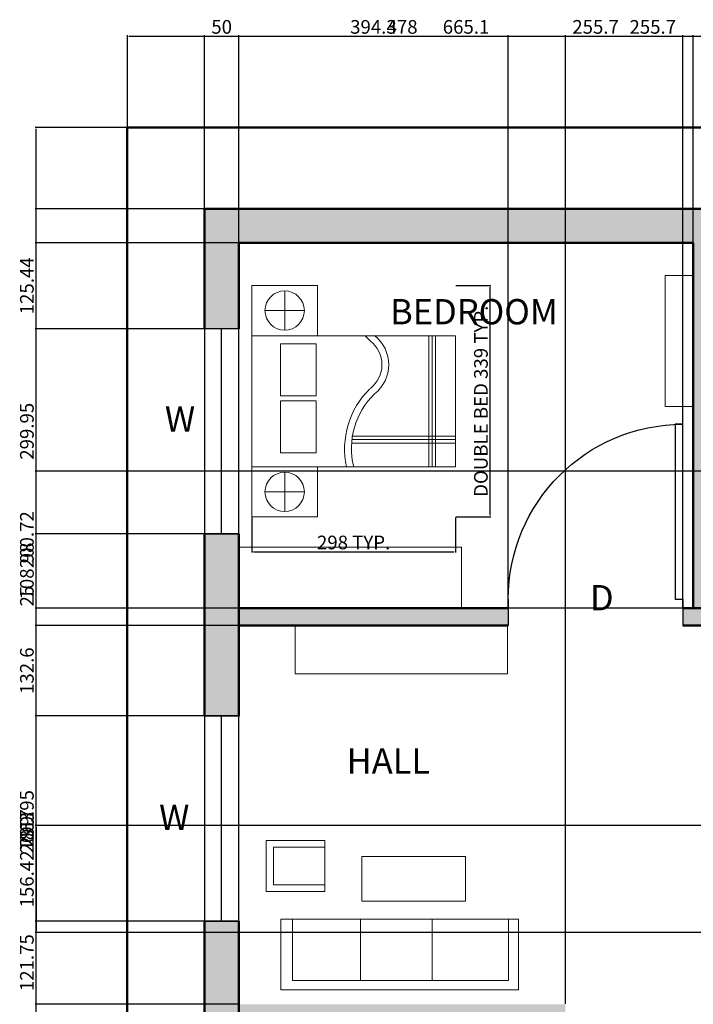
# Model space of a CAD drawing. Units: millimetres. Extents: x 1898 to 8115, y 727 to 4291.
# Tile 4 of 7: x 5191 to 6177, y 2277 to 3717. Entities that reach past the tile are written whole.
import ezdxf

# ---------------------------------------------------------------- set-up
doc = ezdxf.new("R2010")
doc.units = ezdxf.units.MM
for name, color, linetype, lineweight in [('A-ANNO-DIMS', 2, 'Continuous', 18), ('A-ANNO-TEXT', 7, 'Continuous', 25), ('A-AREA-IDEN', 3, 'Continuous', 25), ('A-DOOR', 3, 'Continuous', 25), ('A-FURN', 8, 'Continuous', 18), ('A-GLAZ', 4, 'Continuous', 25), ('A-WALL', 7, 'Continuous', 50), ('A-WALL-PATT', 8, 'Continuous', 13)]:
    doc.layers.add(name, color=color, linetype=linetype, lineweight=lineweight)
doc.styles.get("Standard").update_dxf_attribs({"font": 'arial.ttf'})
doc.dimstyles.new('ISO-25', dxfattribs={"dimtxt": 20, "dimasz": 2.5, "dimexe": 1.25, "dimexo": 0.625, "dimtad": 1, "dimtxsty": 'Standard', "dimcen": 2.5, "dimadec": 0, "dimazin": 0, "dimtfac": 1, "dimtmove": 0, "dimatfit": 3, "dimfxl": 1, "dimarcsym": 0})

# ---------------------------------------------------------------- blocks, each defined once
blk = doc.blocks.new('*U43')
for p, q in [((0, 0), (0, -6)), ((40, 0), (40, -6))]:
    blk.add_line(p, q)
blk.add_lwpolyline([(0, 0), (0, 40), (1.75, 40), (1.75, 0)], close=True)
blk.add_arc((0, 0), 40, 0, 90)
blk = doc.blocks.new('BED-DOUBLE-SET')
for p, q in [((5578.8, 3262.9), (5578.8, 3320.5)), ((5550, 3291.7), (5607.6, 3291.7)), ((5704.8, 3246.7), (5696.6, 3255)), ((5789.5, 3063.1), (5789.5, 3255)), ((5794.5, 3063.1), (5794.5, 3255)), ((5799.5, 3063.1), (5799.5, 3255)), ((5677.2, 3107.9), (5828.6, 3107.9)), ((5677.2, 3102.9), (5828.6, 3102.9)), ((5677.2, 3097.9), (5828.6, 3097.9)), ((5578.8, 2997.7), (5578.8, 3055.3)), ((5550, 3026.5), (5607.6, 3026.5))]:
    blk.add_line(p, q)
for points in [[(5530.8, 3255), (5626.9, 3255), (5626.9, 3328.4), (5530.8, 3328.4)], [(5530.8, 3255), (5828.6, 3255), (5828.6, 3063.1), (5530.8, 3063.1)], [(5572.7, 3167.2), (5624.7, 3167.2), (5624.7, 3243.2), (5572.7, 3243.2)], [(5572.7, 3083.7), (5624.7, 3083.7), (5624.7, 3159.7), (5572.7, 3159.7)], [(5530.8, 2989.8), (5626.9, 2989.8), (5626.9, 3063.1), (5530.8, 3063.1)]]:
    blk.add_lwpolyline(points, close=True)
for centre in [(5578.8, 3291.7), (5578.8, 3026.5)]:
    blk.add_circle(centre, 28.8)
for centre, radius, start, end in [((5677.1, 3212.5), 54, 307.9745, 52.0255), ((5677.1, 3212.5), 44, 307.9745, 52.0255), ((5787.6, 3090), 121.1, 134.0052, 192.8109), ((5787.6, 3090), 111.1, 134.0052, 193.986)]:
    blk.add_arc(centre, radius, start, end)
blk = doc.blocks.new('SOFA-3SEAT')
for p, q in [((6339.2, 3143.3), (6339.2, 3232.9)), ((6339.2, 3232.9), (6655, 3232.9)), ((6438.4, 3232.9), (6438.4, 3143.3)), ((6543.3, 3232.9), (6543.3, 3143.3)), ((6655, 3232.9), (6655, 3143.3))]:
    blk.add_line(p, q)
blk.add_lwpolyline([(6322.2, 3246.6), (6669.9, 3246.6), (6669.9, 3143.3), (6322.2, 3143.3)], close=True)
blk = doc.blocks.new('*D53')
at = {"layer": 'A-ANNO-DIMS', "color": 0, "lineweight": -2, "transparency": 16777216}
for p, q in [((5829.3, 3328.4), (5880.7, 3328.4)), ((5879.4, 2992.3), (5879.4, 3325.9)), ((5829.3, 2989.8), (5880.7, 2989.8))]:
    blk.add_line(p, q, dxfattribs=at)
at = {"layer": 'A-ANNO-DIMS', "color": 0, "transparency": 16777216}
for points in [[(5879, 3325.9), (5879.8, 3325.9), (5879.4, 3328.4)], [(5879, 2992.3), (5879.8, 2992.3), (5879.4, 2989.8)]]:
    blk.add_solid(points, dxfattribs=at)
at = {"layer": 'Defpoints', "color": 0, "transparency": 16777216}
for p in [(5828.6, 3328.4), (5879.4, 3328.4), (5828.6, 2989.8)]:
    blk.add_point(p, dxfattribs=at)
at = {"layer": 'A-ANNO-DIMS', "color": 0, "transparency": 16777216, "insert": (5868.5, 3159.1), "char_height": 20, "attachment_point": 5, "rotation": 90}
blk.add_mtext('DOUBLE BED 339 TYP.', dxfattribs=at)
blk = doc.blocks.new('*D54')
at = {"layer": 'A-ANNO-DIMS', "color": 0, "lineweight": -2, "transparency": 16777216}
for p, q in [((5530.8, 2989.2), (5530.8, 2937.8)), ((5828.6, 2989.2), (5828.6, 2937.8)), ((5533.3, 2939), (5826.1, 2939))]:
    blk.add_line(p, q, dxfattribs=at)
at = {"layer": 'A-ANNO-DIMS', "color": 0, "transparency": 16777216}
for points in [[(5533.3, 2939.4), (5533.3, 2938.6), (5530.8, 2939)], [(5826.1, 2939.4), (5826.1, 2938.6), (5828.6, 2939)]]:
    blk.add_solid(points, dxfattribs=at)
at = {"layer": 'Defpoints', "color": 0, "transparency": 16777216}
for p in [(5530.8, 2989.8), (5828.6, 2989.8), (5828.6, 2939)]:
    blk.add_point(p, dxfattribs=at)
at = {"layer": 'A-ANNO-DIMS', "color": 0, "transparency": 16777216, "insert": (5679.7, 2949.9), "char_height": 20, "attachment_point": 5}
blk.add_mtext('298 TYP.', dxfattribs=at)
blk = doc.blocks.new('*D57')
at = {"layer": 'A-ANNO-DIMS', "color": 0, "lineweight": -2, "transparency": 16777216}
for p, q in [((5348.6, 3560.4), (5348.6, 3694.5)), ((5351.1, 3693.2), (7696.3, 3693.2)), ((7698.8, 3560.4), (7698.8, 3694.5))]:
    blk.add_line(p, q, dxfattribs=at)
at = {"layer": 'A-ANNO-DIMS', "color": 0, "transparency": 16777216}
for points in [[(5351.1, 3693.7), (5351.1, 3692.8), (5348.6, 3693.2)], [(7696.3, 3693.7), (7696.3, 3692.8), (7698.8, 3693.2)]]:
    blk.add_solid(points, dxfattribs=at)
at = {"layer": 'Defpoints', "color": 0, "transparency": 16777216}
for p in [(7698.8, 3693.2), (5348.6, 3559.7), (7698.8, 3559.7)]:
    blk.add_point(p, dxfattribs=at)
at = {"layer": 'A-ANNO-DIMS', "color": 0, "transparency": 16777216, "insert": (6523.7, 3704.1), "char_height": 20, "attachment_point": 5}
blk.add_mtext('2350', dxfattribs=at)
blk = doc.blocks.new('*D58')
at = {"layer": 'A-ANNO-DIMS', "color": 0, "lineweight": -2, "transparency": 16777216}
for p, q in [((5461.6, 3441.3), (5461.6, 3694.5)), ((5464.1, 3693.2), (7567.7, 3693.2)), ((7570.2, 3441.3), (7570.2, 3694.5))]:
    blk.add_line(p, q, dxfattribs=at)
at = {"layer": 'A-ANNO-DIMS', "color": 0, "transparency": 16777216}
for points in [[(5464.1, 3693.7), (5464.1, 3692.8), (5461.6, 3693.2)], [(7567.7, 3693.7), (7567.7, 3692.8), (7570.2, 3693.2)]]:
    blk.add_solid(points, dxfattribs=at)
at = {"layer": 'Defpoints', "color": 0, "transparency": 16777216}
for p in [(7570.2, 3693.2), (5461.6, 3440.7), (7570.2, 3440.7)]:
    blk.add_point(p, dxfattribs=at)
at = {"layer": 'A-ANNO-DIMS', "color": 0, "transparency": 16777216, "insert": (6515.9, 3704.1), "char_height": 20, "attachment_point": 5}
blk.add_mtext('2108.6', dxfattribs=at)
blk = doc.blocks.new('*D59')
at = {"layer": 'A-ANNO-DIMS', "color": 0, "lineweight": -2, "transparency": 16777216}
for p, q in [((5347.9, 3559.7), (5213.8, 3559.7)), ((5215.1, 1499), (5215.1, 3557.2)), ((5347.9, 1496.5), (5213.8, 1496.5))]:
    blk.add_line(p, q, dxfattribs=at)
at = {"layer": 'A-ANNO-DIMS', "color": 0, "transparency": 16777216}
for points in [[(5214.6, 3557.2), (5215.5, 3557.2), (5215.1, 3559.7)], [(5214.6, 1499), (5215.5, 1499), (5215.1, 1496.5)]]:
    blk.add_solid(points, dxfattribs=at)
at = {"layer": 'Defpoints', "color": 0, "transparency": 16777216}
for p in [(5215.1, 3559.7), (5348.6, 3559.7), (5348.6, 1496.5)]:
    blk.add_point(p, dxfattribs=at)
at = {"layer": 'A-ANNO-DIMS', "color": 0, "transparency": 16777216, "insert": (5204.2, 2528.1), "char_height": 20, "attachment_point": 5, "rotation": 90}
blk.add_mtext('2063', dxfattribs=at)
blk = doc.blocks.new('*D60')
at = {"layer": 'A-ANNO-DIMS', "color": 0, "lineweight": -2, "transparency": 16777216}
for p, q in [((5461, 3440.7), (5213.8, 3440.7)), ((5215.1, 1626.1), (5215.1, 3438.2)), ((5461, 1623.6), (5213.8, 1623.6))]:
    blk.add_line(p, q, dxfattribs=at)
at = {"layer": 'A-ANNO-DIMS', "color": 0, "transparency": 16777216}
for points in [[(5214.6, 3438.2), (5215.5, 3438.2), (5215.1, 3440.7)], [(5214.6, 1626.1), (5215.5, 1626.1), (5215.1, 1623.6)]]:
    blk.add_solid(points, dxfattribs=at)
at = {"layer": 'Defpoints', "color": 0, "transparency": 16777216}
for p in [(5215.1, 3440.7), (5461.6, 3440.7), (5461.6, 1623.6)]:
    blk.add_point(p, dxfattribs=at)
at = {"layer": 'A-ANNO-DIMS', "color": 0, "transparency": 16777216, "insert": (5204.2, 2532.1), "char_height": 20, "attachment_point": 5, "rotation": 90}
blk.add_mtext('1817', dxfattribs=at)
blk = doc.blocks.new('*D63')
at = {"layer": 'A-ANNO-DIMS', "color": 0, "lineweight": -2, "transparency": 16777216}
for p, q in [((5461.6, 3265.8), (5461.6, 3694.5)), ((5464.1, 3693.2), (5509.1, 3693.2)), ((5511.6, 3391.3), (5511.6, 3694.5))]:
    blk.add_line(p, q, dxfattribs=at)
at = {"layer": 'A-ANNO-DIMS', "color": 0, "transparency": 16777216}
for points in [[(5464.1, 3693.7), (5464.1, 3692.8), (5461.6, 3693.2)], [(5509.1, 3693.7), (5509.1, 3692.8), (5511.6, 3693.2)]]:
    blk.add_solid(points, dxfattribs=at)
at = {"layer": 'Defpoints', "color": 0, "transparency": 16777216}
for p in [(5511.6, 3693.2), (5511.6, 3390.7), (5461.6, 3265.2)]:
    blk.add_point(p, dxfattribs=at)
at = {"layer": 'A-ANNO-DIMS', "color": 0, "transparency": 16777216, "insert": (5486.6, 3704.1), "char_height": 20, "attachment_point": 5}
blk.add_mtext('50', dxfattribs=at)
blk = doc.blocks.new('*D64')
at = {"layer": 'A-ANNO-DIMS', "color": 0, "lineweight": -2, "transparency": 16777216}
for p, q in [((5511.6, 3391.3), (5511.6, 3694.5)), ((5514.1, 3693.2), (6174.2, 3693.2)), ((6176.7, 3391.3), (6176.7, 3694.5))]:
    blk.add_line(p, q, dxfattribs=at)
at = {"layer": 'A-ANNO-DIMS', "color": 0, "transparency": 16777216}
for points in [[(5514.1, 3693.7), (5514.1, 3692.8), (5511.6, 3693.2)], [(6174.2, 3693.7), (6174.2, 3692.8), (6176.7, 3693.2)]]:
    blk.add_solid(points, dxfattribs=at)
at = {"layer": 'Defpoints', "color": 0, "transparency": 16777216}
for p in [(6176.7, 3693.2), (5511.6, 3390.7), (6176.7, 3390.7)]:
    blk.add_point(p, dxfattribs=at)
at = {"layer": 'A-ANNO-DIMS', "color": 0, "transparency": 16777216, "insert": (5844.2, 3704.1), "char_height": 20, "attachment_point": 5}
blk.add_mtext('665.1', dxfattribs=at)
blk = doc.blocks.new('*D83')
at = {"layer": 'A-ANNO-DIMS', "color": 0, "lineweight": -2, "transparency": 16777216}
for p, q in [((5511, 2277), (5213.8, 2277)), ((5215.1, 2229.5), (5215.1, 2274.5)), ((5511, 2227), (5213.8, 2227))]:
    blk.add_line(p, q, dxfattribs=at)
at = {"layer": 'A-ANNO-DIMS', "color": 0, "transparency": 16777216}
for points in [[(5214.6, 2274.5), (5215.5, 2274.5), (5215.1, 2277)], [(5214.6, 2229.5), (5215.5, 2229.5), (5215.1, 2227)]]:
    blk.add_solid(points, dxfattribs=at)
at = {"layer": 'Defpoints', "color": 0, "transparency": 16777216}
for p in [(5215.1, 2277), (5511.6, 2277), (5511.6, 2227)]:
    blk.add_point(p, dxfattribs=at)
at = {"layer": 'A-ANNO-DIMS', "color": 0, "transparency": 16777216, "insert": (5204.2, 2252), "char_height": 20, "attachment_point": 5, "rotation": 90}
blk.add_mtext('50', dxfattribs=at)
blk = doc.blocks.new('*D84')
at = {"layer": 'A-ANNO-DIMS', "color": 0, "lineweight": -2, "transparency": 16777216}
for p, q in [((5511, 2398.7), (5213.8, 2398.7)), ((5215.1, 2279.5), (5215.1, 2396.2)), ((5511, 2277), (5213.8, 2277))]:
    blk.add_line(p, q, dxfattribs=at)
at = {"layer": 'A-ANNO-DIMS', "color": 0, "transparency": 16777216}
for points in [[(5214.6, 2396.2), (5215.5, 2396.2), (5215.1, 2398.7)], [(5214.6, 2279.5), (5215.5, 2279.5), (5215.1, 2277)]]:
    blk.add_solid(points, dxfattribs=at)
at = {"layer": 'Defpoints', "color": 0, "transparency": 16777216}
for p in [(5215.1, 2398.7), (5511.6, 2398.7), (5511.6, 2277)]:
    blk.add_point(p, dxfattribs=at)
at = {"layer": 'A-ANNO-DIMS', "color": 0, "transparency": 16777216, "insert": (5204.2, 2337.9), "char_height": 20, "attachment_point": 5, "rotation": 90}
blk.add_mtext('121.75', dxfattribs=at)
blk = doc.blocks.new('*D85')
at = {"layer": 'A-ANNO-DIMS', "color": 0, "lineweight": -2, "transparency": 16777216}
for p, q in [((5511, 2698.7), (5213.8, 2698.7)), ((5215.1, 2401.2), (5215.1, 2696.2)), ((5511, 2398.7), (5213.8, 2398.7))]:
    blk.add_line(p, q, dxfattribs=at)
at = {"layer": 'A-ANNO-DIMS', "color": 0, "transparency": 16777216}
for points in [[(5214.6, 2696.2), (5215.5, 2696.2), (5215.1, 2698.7)], [(5214.6, 2401.2), (5215.5, 2401.2), (5215.1, 2398.7)]]:
    blk.add_solid(points, dxfattribs=at)
at = {"layer": 'Defpoints', "color": 0, "transparency": 16777216}
for p in [(5215.1, 2698.7), (5511.6, 2698.7), (5511.6, 2398.7)]:
    blk.add_point(p, dxfattribs=at)
at = {"layer": 'A-ANNO-DIMS', "color": 0, "transparency": 16777216, "insert": (5204.2, 2548.7), "char_height": 20, "attachment_point": 5, "rotation": 90}
blk.add_mtext('299.95', dxfattribs=at)
blk = doc.blocks.new('*D86')
at = {"layer": 'A-ANNO-DIMS', "color": 0, "lineweight": -2, "transparency": 16777216}
for p, q in [((5511, 2831.3), (5213.8, 2831.3)), ((5215.1, 2701.2), (5215.1, 2828.8)), ((5511, 2698.7), (5213.8, 2698.7))]:
    blk.add_line(p, q, dxfattribs=at)
at = {"layer": 'A-ANNO-DIMS', "color": 0, "transparency": 16777216}
for points in [[(5214.6, 2828.8), (5215.5, 2828.8), (5215.1, 2831.3)], [(5214.6, 2701.2), (5215.5, 2701.2), (5215.1, 2698.7)]]:
    blk.add_solid(points, dxfattribs=at)
at = {"layer": 'Defpoints', "color": 0, "transparency": 16777216}
for p in [(5215.1, 2831.3), (5511.6, 2831.3), (5511.6, 2698.7)]:
    blk.add_point(p, dxfattribs=at)
at = {"layer": 'A-ANNO-DIMS', "color": 0, "transparency": 16777216, "insert": (5204.2, 2765), "char_height": 20, "attachment_point": 5, "rotation": 90}
blk.add_mtext('132.6', dxfattribs=at)
blk = doc.blocks.new('*D87')
at = {"layer": 'A-ANNO-DIMS', "color": 0, "lineweight": -2, "transparency": 16777216}
for p, q in [((5215.1, 2856.3), (5215.1, 2889.2)), ((5511, 2856.3), (5213.8, 2856.3)), ((5215.1, 2833.8), (5215.1, 2853.8)), ((5511, 2831.3), (5213.8, 2831.3))]:
    blk.add_line(p, q, dxfattribs=at)
at = {"layer": 'A-ANNO-DIMS', "color": 0, "transparency": 16777216}
for points in [[(5214.6, 2853.8), (5215.5, 2853.8), (5215.1, 2856.3)], [(5214.6, 2833.8), (5215.5, 2833.8), (5215.1, 2831.3)]]:
    blk.add_solid(points, dxfattribs=at)
at = {"layer": 'Defpoints', "color": 0, "transparency": 16777216}
for p in [(5215.1, 2856.3), (5511.6, 2856.3), (5511.6, 2831.3)]:
    blk.add_point(p, dxfattribs=at)
at = {"layer": 'A-ANNO-DIMS', "color": 0, "transparency": 16777216, "insert": (5204.2, 2874), "char_height": 20, "attachment_point": 5, "rotation": 90}
blk.add_mtext('25', dxfattribs=at)
blk = doc.blocks.new('*D88')
at = {"layer": 'A-ANNO-DIMS', "color": 0, "lineweight": -2, "transparency": 16777216}
for p, q in [((5511, 2965.3), (5213.8, 2965.3)), ((5215.1, 2858.8), (5215.1, 2962.8)), ((5511, 2856.3), (5213.8, 2856.3))]:
    blk.add_line(p, q, dxfattribs=at)
at = {"layer": 'A-ANNO-DIMS', "color": 0, "transparency": 16777216}
for points in [[(5214.6, 2962.8), (5215.5, 2962.8), (5215.1, 2965.3)], [(5214.6, 2858.8), (5215.5, 2858.8), (5215.1, 2856.3)]]:
    blk.add_solid(points, dxfattribs=at)
at = {"layer": 'Defpoints', "color": 0, "transparency": 16777216}
for p in [(5215.1, 2965.3), (5511.6, 2965.3), (5511.6, 2856.3)]:
    blk.add_point(p, dxfattribs=at)
at = {"layer": 'A-ANNO-DIMS', "color": 0, "transparency": 16777216, "insert": (5204.2, 2910.8), "char_height": 20, "attachment_point": 5, "rotation": 90}
blk.add_mtext('108.98', dxfattribs=at)
blk = doc.blocks.new('*D89')
at = {"layer": 'A-ANNO-DIMS', "color": 0, "lineweight": -2, "transparency": 16777216}
for p, q in [((5511, 3265.2), (5213.8, 3265.2)), ((5215.1, 2967.8), (5215.1, 3262.7)), ((5511, 2965.3), (5213.8, 2965.3))]:
    blk.add_line(p, q, dxfattribs=at)
at = {"layer": 'A-ANNO-DIMS', "color": 0, "transparency": 16777216}
for points in [[(5214.6, 3262.7), (5215.5, 3262.7), (5215.1, 3265.2)], [(5214.6, 2967.8), (5215.5, 2967.8), (5215.1, 2965.3)]]:
    blk.add_solid(points, dxfattribs=at)
at = {"layer": 'Defpoints', "color": 0, "transparency": 16777216}
for p in [(5215.1, 3265.2), (5511.6, 3265.2), (5511.6, 2965.3)]:
    blk.add_point(p, dxfattribs=at)
at = {"layer": 'A-ANNO-DIMS', "color": 0, "transparency": 16777216, "insert": (5204.2, 3115.2), "char_height": 20, "attachment_point": 5, "rotation": 90}
blk.add_mtext('299.95', dxfattribs=at)
blk = doc.blocks.new('*D90')
at = {"layer": 'A-ANNO-DIMS', "color": 0, "lineweight": -2, "transparency": 16777216}
for p, q in [((5511, 3390.7), (5213.8, 3390.7)), ((5215.1, 3267.7), (5215.1, 3388.2)), ((5511, 3265.2), (5213.8, 3265.2))]:
    blk.add_line(p, q, dxfattribs=at)
at = {"layer": 'A-ANNO-DIMS', "color": 0, "transparency": 16777216}
for points in [[(5214.6, 3388.2), (5215.5, 3388.2), (5215.1, 3390.7)], [(5214.6, 3267.7), (5215.5, 3267.7), (5215.1, 3265.2)]]:
    blk.add_solid(points, dxfattribs=at)
at = {"layer": 'Defpoints', "color": 0, "transparency": 16777216}
for p in [(5215.1, 3390.7), (5511.6, 3390.7), (5511.6, 3265.2)]:
    blk.add_point(p, dxfattribs=at)
at = {"layer": 'A-ANNO-DIMS', "color": 0, "transparency": 16777216, "insert": (5204.2, 3327.9), "char_height": 20, "attachment_point": 5, "rotation": 90}
blk.add_mtext('125.44', dxfattribs=at)
blk = doc.blocks.new('*D103')
at = {"layer": 'A-ANNO-DIMS', "color": 0, "lineweight": -2, "transparency": 16777216}
for p, q in [((5511.6, 2856.9), (5511.6, 3694.5)), ((5514.1, 3693.2), (5903.4, 3693.2)), ((5905.9, 2856.9), (5905.9, 3694.5))]:
    blk.add_line(p, q, dxfattribs=at)
at = {"layer": 'A-ANNO-DIMS', "color": 0, "transparency": 16777216}
for points in [[(5514.1, 3693.7), (5514.1, 3692.8), (5511.6, 3693.2)], [(5903.4, 3693.7), (5903.4, 3692.8), (5905.9, 3693.2)]]:
    blk.add_solid(points, dxfattribs=at)
at = {"layer": 'Defpoints', "color": 0, "transparency": 16777216}
for p in [(5905.9, 3693.2), (5511.6, 2856.3), (5905.9, 2856.3)]:
    blk.add_point(p, dxfattribs=at)
at = {"layer": 'A-ANNO-DIMS', "color": 0, "transparency": 16777216, "insert": (5708.7, 3704.1), "char_height": 20, "attachment_point": 5}
blk.add_mtext('394.3', dxfattribs=at)
blk = doc.blocks.new('*D104')
at = {"layer": 'A-ANNO-DIMS', "color": 0, "lineweight": -2, "transparency": 16777216}
for p, q in [((5905.9, 2856.9), (5905.9, 3694.5)), ((5908.4, 3693.2), (6159.1, 3693.2)), ((6161.6, 2856.9), (6161.6, 3694.5))]:
    blk.add_line(p, q, dxfattribs=at)
at = {"layer": 'A-ANNO-DIMS', "color": 0, "transparency": 16777216}
for points in [[(5908.4, 3693.7), (5908.4, 3692.8), (5905.9, 3693.2)], [(6159.1, 3693.7), (6159.1, 3692.8), (6161.6, 3693.2)]]:
    blk.add_solid(points, dxfattribs=at)
at = {"layer": 'Defpoints', "color": 0, "transparency": 16777216}
for p in [(6161.6, 3693.2), (5905.9, 2856.3), (6161.6, 2856.3)]:
    blk.add_point(p, dxfattribs=at)
at = {"layer": 'A-ANNO-DIMS', "color": 0, "transparency": 16777216, "insert": (6033.7, 3704.1), "char_height": 20, "attachment_point": 5}
blk.add_mtext('255.7', dxfattribs=at)
blk = doc.blocks.new('*D105')
at = {"layer": 'A-ANNO-DIMS', "color": 0, "lineweight": -2, "transparency": 16777216}
for p, q in [((5511.6, 2277.6), (5511.6, 3694.5)), ((5514.1, 3693.2), (5987.1, 3693.2)), ((5989.6, 2277.6), (5989.6, 3694.5))]:
    blk.add_line(p, q, dxfattribs=at)
at = {"layer": 'A-ANNO-DIMS', "color": 0, "transparency": 16777216}
for points in [[(5514.1, 3693.7), (5514.1, 3692.8), (5511.6, 3693.2)], [(5987.1, 3693.7), (5987.1, 3692.8), (5989.6, 3693.2)]]:
    blk.add_solid(points, dxfattribs=at)
at = {"layer": 'Defpoints', "color": 0, "transparency": 16777216}
for p in [(5989.6, 3693.2), (5511.6, 2277), (5989.6, 2277)]:
    blk.add_point(p, dxfattribs=at)
at = {"layer": 'A-ANNO-DIMS', "color": 0, "transparency": 16777216, "insert": (5750.6, 3704.1), "char_height": 20, "attachment_point": 5}
blk.add_mtext('478', dxfattribs=at)
blk = doc.blocks.new('*D106')
at = {"layer": 'A-ANNO-DIMS', "color": 0, "lineweight": -2, "transparency": 16777216}
for p, q in [((5989.6, 2277.6), (5989.6, 3694.5)), ((5992.1, 3693.2), (6242.8, 3693.2)), ((6245.3, 2277.6), (6245.3, 3694.5))]:
    blk.add_line(p, q, dxfattribs=at)
at = {"layer": 'A-ANNO-DIMS', "color": 0, "transparency": 16777216}
for points in [[(5992.1, 3693.7), (5992.1, 3692.8), (5989.6, 3693.2)], [(6242.8, 3693.7), (6242.8, 3692.8), (6245.3, 3693.2)]]:
    blk.add_solid(points, dxfattribs=at)
at = {"layer": 'Defpoints', "color": 0, "transparency": 16777216}
for p in [(6245.3, 3693.2), (5989.6, 2277), (6245.3, 2277)]:
    blk.add_point(p, dxfattribs=at)
at = {"layer": 'A-ANNO-DIMS', "color": 0, "transparency": 16777216, "insert": (6117.4, 3704.1), "char_height": 20, "attachment_point": 5}
blk.add_mtext('255.7', dxfattribs=at)
blk = doc.blocks.new('*D110')
at = {"layer": 'A-ANNO-DIMS', "color": 0, "lineweight": -2, "transparency": 16777216}
for p, q in [((6809.3, 3057), (5213.8, 3057)), ((5215.1, 2858.8), (5215.1, 3054.5)), ((6809.3, 2856.3), (5213.8, 2856.3))]:
    blk.add_line(p, q, dxfattribs=at)
at = {"layer": 'A-ANNO-DIMS', "color": 0, "transparency": 16777216}
for points in [[(5214.6, 3054.5), (5215.5, 3054.5), (5215.1, 3057)], [(5214.6, 2858.8), (5215.5, 2858.8), (5215.1, 2856.3)]]:
    blk.add_solid(points, dxfattribs=at)
at = {"layer": 'Defpoints', "color": 0, "transparency": 16777216}
for p in [(5215.1, 3057), (6809.9, 3057), (6809.9, 2856.3)]:
    blk.add_point(p, dxfattribs=at)
at = {"layer": 'A-ANNO-DIMS', "color": 0, "transparency": 16777216, "insert": (5204.2, 2956.6), "char_height": 20, "attachment_point": 5, "rotation": 90}
blk.add_mtext('200.72', dxfattribs=at)
blk = doc.blocks.new('*D113')
at = {"layer": 'A-ANNO-DIMS', "color": 0, "lineweight": -2, "transparency": 16777216}
for p, q in [((6965.2, 2538.5), (5213.8, 2538.5)), ((5215.1, 2536), (5215.1, 2384.6)), ((6965.2, 2382.1), (5213.8, 2382.1))]:
    blk.add_line(p, q, dxfattribs=at)
at = {"layer": 'A-ANNO-DIMS', "color": 0, "transparency": 16777216}
for points in [[(5214.6, 2536), (5215.5, 2536), (5215.1, 2538.5)], [(5214.6, 2384.6), (5215.5, 2384.6), (5215.1, 2382.1)]]:
    blk.add_solid(points, dxfattribs=at)
at = {"layer": 'Defpoints', "color": 0, "transparency": 16777216}
for p in [(6965.8, 2538.5), (5215.1, 2382.1), (6965.8, 2382.1)]:
    blk.add_point(p, dxfattribs=at)
at = {"layer": 'A-ANNO-DIMS', "color": 0, "transparency": 16777216, "insert": (5204.2, 2460.3), "char_height": 20, "attachment_point": 5, "rotation": 90}
blk.add_mtext('156.42', dxfattribs=at)

msp = doc.modelspace()

# ---------------------------------------------------------------- hatches: boundary and pattern name
at = {"layer": 'A-WALL-PATT'}
h = msp.add_hatch(color=256, dxfattribs=at)
h.dxf.hatch_style = 1
h.paths.add_polyline_path([(6201.726, 3440.661), (5461.585, 3440.661), (5461.585, 3265.221), (5511.585, 3265.221), (5511.585, 3390.661), (6176.726, 3390.661), (6176.726, 2856.284), (6201.726, 2856.284)])
h.paths.add_polyline_path([(6784.895, 3318.017), (6201.726, 3318.017), (6201.726, 3268.017), (6784.895, 3268.017)])
h.paths.add_polyline_path([(7570.217, 3440.661), (6784.895, 3440.661), (6784.895, 3057.009), (6809.895, 3057.009), (6809.895, 3390.661), (7520.217, 3390.661), (7520.217, 3300.311), (7570.217, 3300.311)])
h.paths.add_polyline_path([(7570.217, 3000.359), (7520.217, 3000.359), (7520.217, 2758.681), (7570.217, 2758.681)])
h.paths.add_polyline_path([(7520.217, 2856.284), (7194.283, 2856.284), (6784.895, 2856.284), (6784.895, 2831.284), (7520.217, 2831.284)])
h.paths.add_polyline_path([(6809.895, 2878.069), (6784.895, 2878.069), (6784.895, 2856.284), (6809.895, 2856.284)])
h.paths.add_polyline_path([(6201.726, 2856.284), (6176.726, 2856.284), (6161.551, 2856.284), (6161.551, 2831.284), (6201.726, 2831.284)])
h.paths.add_polyline_path([(5905.861, 2856.284), (5511.585, 2856.284), (5511.585, 2831.284), (5905.861, 2831.284)])
h.paths.add_polyline_path([(5511.585, 2965.269), (5461.585, 2965.269), (5461.585, 2698.678), (5511.585, 2698.678)])
h.paths.add_polyline_path([(5511.585, 2398.725), (5461.585, 2398.725), (5461.585, 2088.028), (5511.585, 2088.028)])
h.paths.add_polyline_path([(5989.6, 2238.621), (5989.6, 2276.975), (5511.585, 2276.975), (5511.585, 2226.975), (5989.865, 2226.975, -0.01139164)])
h.paths.add_polyline_path([(6636.013, 2276.975), (6245.29, 2276.975), (6245.29, 2238.621), (6245.29, 2226.975), (6636.013, 2226.975), (6636.013, 2238.621)])
h.paths.add_polyline_path([(7570.217, 2359.481), (7520.217, 2359.481), (7520.217, 2326.802), (7520.217, 2276.975), (6891.704, 2276.975), (6891.704, 2238.621, -0.01139164), (6891.439, 2226.975), (7570.217, 2226.975)])
h.paths.add_polyline_path([(7145.586, 2531.644), (6989.313, 2531.644), (6989.313, 2538.488), (7145.735, 2538.488), (7145.735, 2531.644), (7145.586, 2531.644, -0.39860379), (6990.849, 2382.073), (6990.849, 2276.975), (6965.849, 2276.975), (6965.849, 2382.065), (6989.313, 2382.065, 0.40145271)])
h.paths.add_polyline_path([(6990.849, 2596.561), (6989.313, 2596.561), (6965.849, 2596.561), (6965.849, 2538.488), (6990.849, 2538.488)])
h.paths.add_polyline_path([(6990.849, 2831.284), (6965.849, 2831.284), (6965.849, 2752.984), (6990.849, 2752.984)])
h.paths.add_polyline_path([(7570.217, 2638.517), (7520.217, 2638.517), (7520.217, 2625.002), (7520.217, 2479.644), (7570.217, 2479.644)])
h.paths.add_polyline_path([(7520.217, 2579.13), (6990.849, 2579.13), (6990.849, 2554.13), (7520.217, 2554.13)])

# ---------------------------------------------------------------- linework, layer by layer
at = {"layer": 'A-FURN'}
for p, q in [((5562.41, 2451.944), (5562.41, 2506.773)), ((5562.41, 2506.773), (5637.567, 2506.773)), ((5637.567, 2451.944), (5562.41, 2451.944))]:
    msp.add_line(p, q, dxfattribs=at)
for points in [[(6176.726, 3151.538), (6135.505, 3151.538), (6135.505, 3343.263), (6176.726, 3343.263)], [(5511.585, 2856.284), (5837.518, 2856.284), (5837.518, 2945.821), (5511.585, 2945.821)], [(5594.049, 2831.284), (5904.749, 2831.284), (5904.749, 2760.228), (5594.049, 2760.228)], [(5637.567, 2442.127), (5551.653, 2442.127), (5551.653, 2516.579), (5637.567, 2516.579)], [(5691.592, 2493.226), (5843.572, 2493.226), (5843.572, 2428.022), (5691.592, 2428.022)]]:
    msp.add_lwpolyline(points, close=True, dxfattribs=at)
at = {"layer": 'A-GLAZ'}
for p, q in [((5486.585, 2965.269), (5486.585, 3265.221)), ((5486.585, 2398.725), (5486.585, 2698.678))]:
    msp.add_line(p, q, dxfattribs=at)
for points in [[(5511.585, 3265.221), (5461.585, 3265.221)], [(5461.585, 2965.269), (5511.585, 2965.269)], [(5511.585, 2698.678), (5461.585, 2698.678)], [(5461.585, 2398.725), (5511.585, 2398.725)]]:
    msp.add_lwpolyline(points, dxfattribs=at)
for points in [[(5461.585, 2965.269), (5511.585, 2965.269), (5511.585, 3265.221), (5461.585, 3265.221)], [(5511.585, 2698.678), (5461.585, 2698.678), (5461.585, 2398.725), (5511.585, 2398.725)]]:
    msp.add_lwpolyline(points, close=True, dxfattribs=at)
at = {"layer": 'A-WALL'}
for p, q in [((5461.585, 3440.661), (6201.726, 3440.661)), ((5461.585, 3265.221), (5461.585, 3440.661)), ((5511.585, 3390.661), (6176.726, 3390.661)), ((5511.585, 3265.221), (5511.585, 3390.661)), ((6176.726, 3390.661), (6176.726, 2856.284)), ((5461.585, 2698.678), (5461.585, 2965.269)), ((5511.585, 2698.678), (5511.585, 2965.269)), ((5511.585, 2856.284), (5905.861, 2856.284)), ((6161.551, 2856.284), (6201.726, 2856.284)), ((5511.585, 2831.284), (5905.861, 2831.284)), ((6161.551, 2831.284), (6201.726, 2831.284)), ((5461.585, 2088.028), (5461.585, 2398.725)), ((5511.585, 2088.028), (5511.585, 2398.725))]:
    msp.add_line(p, q, dxfattribs=at)
msp.add_lwpolyline([(5348.551, 3559.737), (7698.767, 3559.737), (7698.767, 1496.544), (5348.551, 1496.544)], close=True, dxfattribs=at)

# ---------------------------------------------------------------- block references
at = {"layer": 'A-DOOR', "xscale": -6.392265120440044, "yscale": 6.392265120440044, "zscale": 6.392265120440044}
msp.add_blockref('*U43', (6161.551, 2869.638), dxfattribs=at)
at = {"layer": 'A-FURN'}
msp.add_blockref('BED-DOUBLE-SET', (0, 0), dxfattribs=at)
at = {"layer": 'A-FURN', "extrusion": (0, 0, -1), "zscale": -1, "rotation": 180}
msp.add_blockref('SOFA-3SEAT', (748.869, 5544.782), dxfattribs=at)

# ---------------------------------------------------------------- texts
at = {"layer": 'A-ANNO-TEXT', "char_height": 36.981, "attachment_point": 1}
for s, insert in [('W', (5403.512, 3151.453)), ('D', (6025.451, 2890.227)), ('W', (5395.077, 2568.96))]:
    msp.add_mtext_dynamic_manual_height_columns(s, width=5503.90807, gutter_width=184.907, heights=[0], dxfattribs=dict(at, insert=insert))
at = {"layer": 'A-AREA-IDEN', "char_height": 36.9814, "attachment_point": 1}
for s, insert in [('BEDROOM', (5733.085, 3308.532)), ('HALL', (5669.467, 2651.413))]:
    msp.add_mtext_dynamic_manual_height_columns(s, width=5503.90807, gutter_width=184.907, heights=[0], dxfattribs=dict(at, insert=insert))

# ---------------------------------------------------------------- dimensions: what is measured, and where the dimension line sits
at = {"layer": 'A-ANNO-DIMS'}
for base, p1, p2, override, picture, middle in [((7698.767, 3693.237), (5348.551, 3559.737), (7698.767, 3559.737), {"dimdec": 0, "dimlfac": 1, "dimrnd": 0, "dimzin": 0, "dimdsep": 46, "dimlunit": 2}, '*D57', (6523.659, 3704.08)), ((7570.217, 3693.237), (5461.585, 3440.661), (7570.217, 3440.661), {"dimdec": 1, "dimlfac": 1, "dimrnd": 0, "dimzin": 0, "dimdsep": 46, "dimlunit": 2}, '*D58', (6515.901, 3704.073)), ((5511.585, 3693.237), (5461.585, 3265.221), (5511.585, 3390.661), {"dimdec": 0, "dimlfac": 1, "dimrnd": 0, "dimzin": 0, "dimdsep": 46, "dimlunit": 2}, '*D63', (5486.585, 3704.073)), ((5905.861, 3693.237), (5511.585, 2856.284), (5905.861, 2856.284), {"dimdec": 1, "dimlfac": 1, "dimrnd": 0, "dimzin": 0, "dimdsep": 46, "dimlunit": 2}, '*D103', (5708.723, 3704.08)), ((6176.726, 3693.237), (5511.585, 3390.661), (6176.726, 3390.661), {"dimdec": 1, "dimlfac": 1, "dimrnd": 0, "dimzin": 0, "dimdsep": 46, "dimlunit": 2}, '*D64', (5844.155, 3704.073)), ((5989.6, 3693.237), (5511.585, 2276.975), (5989.6, 2276.975), {"dimdec": 0, "dimlfac": 1, "dimrnd": 0, "dimzin": 0, "dimdsep": 46, "dimlunit": 2}, '*D105', (5750.592, 3704.073)), ((6161.551, 3693.237), (5905.861, 2856.284), (6161.551, 2856.284), {"dimdec": 1, "dimlfac": 1, "dimrnd": 0, "dimzin": 0, "dimdsep": 46, "dimlunit": 2}, '*D104', (6033.706, 3704.073)), ((6245.29, 3693.237), (5989.6, 2276.975), (6245.29, 2276.975), {"dimdec": 1, "dimlfac": 1, "dimrnd": 0, "dimzin": 0, "dimdsep": 46, "dimlunit": 2}, '*D106', (6117.445, 3704.073))]:
    dim = msp.add_linear_dim(base=base, p1=p1, p2=p2, dimstyle='ISO-25', override=override, dxfattribs=at)
    dim.commit()
    dim.dimension.update_dxf_attribs({"geometry": picture, "text_midpoint": middle})
for base, p1, p2, override, picture, middle in [((5215.051, 3559.737), (5348.551, 1496.544), (5348.551, 3559.737), {"dimdec": 0, "dimlfac": 1, "dimrnd": 0, "dimzin": 0, "dimdsep": 46, "dimlunit": 2}, '*D59', (5204.207, 2528.14)), ((5215.051, 3440.661), (5461.585, 1623.621), (5461.585, 3440.661), {"dimdec": 0, "dimlfac": 1, "dimrnd": 0, "dimzin": 0, "dimdsep": 46, "dimlunit": 2}, '*D60', (5204.214, 2532.141)), ((5215.051, 3390.661), (5511.585, 3265.221), (5511.585, 3390.661), {"dimdec": 2, "dimlfac": 1, "dimrnd": 0, "dimzin": 0, "dimdsep": 46, "dimlunit": 2}, '*D90', (5204.214, 3327.941)), ((5215.051, 3265.221), (5511.585, 2965.269), (5511.585, 3265.221), {"dimdec": 2, "dimlfac": 1, "dimrnd": 0, "dimzin": 0, "dimdsep": 46, "dimlunit": 2}, '*D89', (5204.214, 3115.245)), ((5215.0506, 3057.0088), (6809.8949, 2856.2845), (6809.8949, 3057.0088), {"dimdec": 2, "dimlfac": 1, "dimrnd": 0, "dimzin": 0, "dimdsep": 46, "dimlunit": 2}, '*D110', (5204.2141, 2956.6467)), ((5215.0506, 2965.2687), (5511.5848, 2856.2845), (5511.5848, 2965.2687), {"dimdec": 2, "dimlfac": 1, "dimrnd": 0, "dimzin": 0, "dimdsep": 46, "dimlunit": 2}, '*D88', (5204.2141, 2910.7766)), ((5215.051, 2856.284), (5511.585, 2831.284), (5511.585, 2856.284), {"dimdec": 0, "dimlfac": 1, "dimrnd": 0, "dimzin": 0, "dimdsep": 46, "dimlunit": 2}, '*D87', (5204.214, 2873.98)), ((5215.051, 2831.284), (5511.585, 2698.678), (5511.585, 2831.284), {"dimdec": 1, "dimlfac": 1, "dimrnd": 0, "dimzin": 0, "dimdsep": 46, "dimlunit": 2}, '*D86', (5204.207, 2764.981)), ((5215.051, 2698.678), (5511.585, 2398.725), (5511.585, 2698.678), {"dimdec": 2, "dimlfac": 1, "dimrnd": 0, "dimzin": 0, "dimdsep": 46, "dimlunit": 2}, '*D85', (5204.214, 2548.701)), ((5215.051, 2382.065), (6965.849, 2538.488), (6965.849, 2382.065), {"dimdec": 2, "dimlfac": 1, "dimrnd": 0, "dimzin": 0, "dimdsep": 46, "dimlunit": 2}, '*D113', (5204.214, 2460.277)), ((5215.051, 2398.725), (5511.585, 2276.975), (5511.585, 2398.725), {"dimdec": 2, "dimlfac": 1, "dimrnd": 0, "dimzin": 0, "dimdsep": 46, "dimlunit": 2}, '*D84', (5204.214, 2337.85)), ((5215.051, 2276.975), (5511.585, 2226.975), (5511.585, 2276.975), {"dimdec": 0, "dimlfac": 1, "dimrnd": 0, "dimzin": 0, "dimdsep": 46, "dimlunit": 2}, '*D83', (5204.214, 2251.975))]:
    dim = msp.add_linear_dim(base=base, p1=p1, p2=p2, angle=90, dimstyle='ISO-25', override=override, dxfattribs=at)
    dim.commit()
    dim.dimension.update_dxf_attribs({"geometry": picture, "text_midpoint": middle})
dim = msp.add_linear_dim(base=(5879.431, 3328.353), p1=(5828.649, 2989.803), p2=(5828.649, 3328.353), angle=90, text='DOUBLE BED <> TYP.', dimstyle='ISO-25', override={"dimdec": 0, "dimrnd": 0, "dimzin": 0, "dimlunit": 2}, dxfattribs=at)
dim.commit()
dim.dimension.update_dxf_attribs({"geometry": '*D53', "text_midpoint": (5868.452, 3159.078)})
dim = msp.add_linear_dim(base=(5828.649, 2939.02), p1=(5530.81, 2989.803), p2=(5828.649, 2989.803), text='<> TYP.', dimstyle='ISO-25', override={"dimdec": 0, "dimrnd": 0, "dimzin": 0, "dimlunit": 2}, dxfattribs=at)
dim.commit()
dim.dimension.update_dxf_attribs({"geometry": '*D54', "text_midpoint": (5679.729, 2949.857)})

doc.saveas('drawing.dxf')
